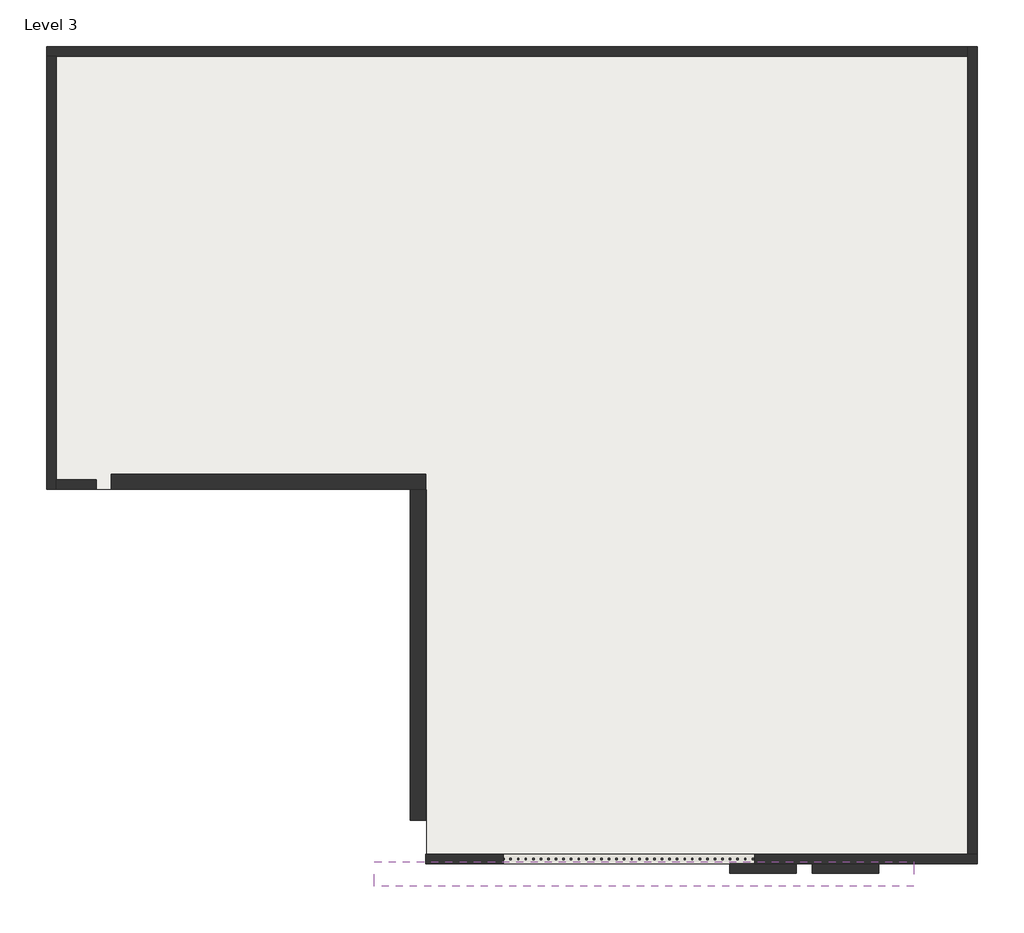
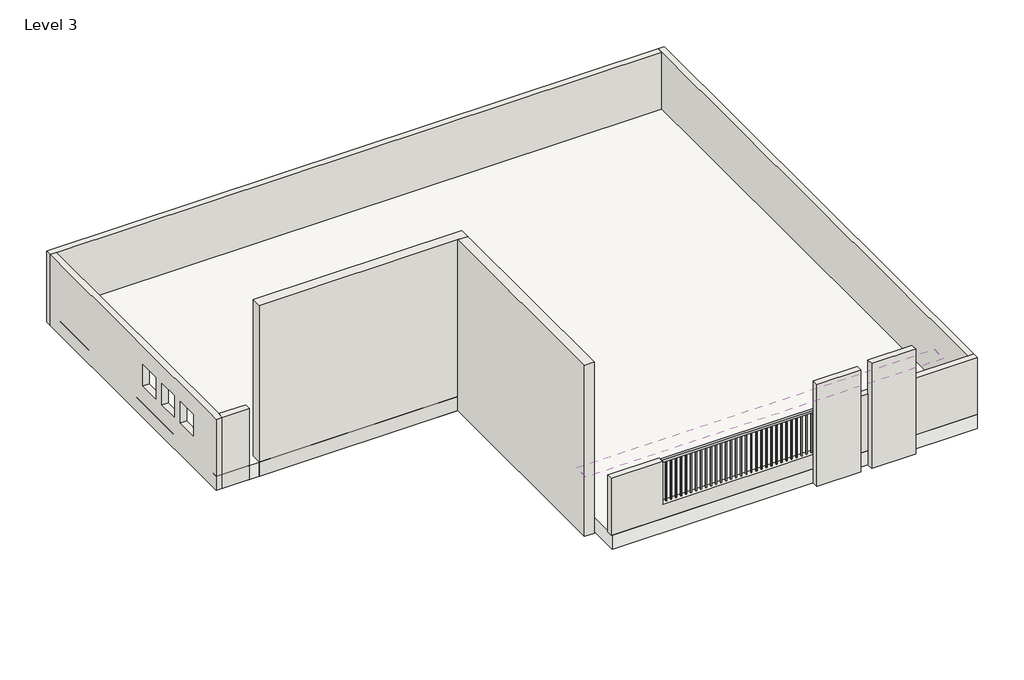
# One storey: 9 walls, 2 roofs, 1 railing.
"""IFC4 building model written with IfcOpenShell, lengths in millimetres."""

from ifc_helpers import new_model, si_unit, frame, origin, place, context, project, spatial, polyline, outline, extrude, faceted_brep, element, save

model = new_model("IFC4")

# Units and contexts
model_context = context("Model", 3, world=origin())
ifc_project = project(units=[si_unit("LENGTHUNIT", "METRE", prefix="MILLI")], contexts=[model_context])

# Site, building, storey
site = spatial("IfcSite", under=ifc_project)
building = spatial("IfcBuilding", under=site)
storey = spatial("IfcBuildingStorey", under=building, Name="Level 3", Elevation=7315.2)

# Railing
placement = place(None, origin())
element("IfcRailing", 1, ObjectType="Handrail - Rectangular", at=placement, inside=storey, context=model_context, shape_type="SweptSolid", body=[
    extrude(outline(polyline([(-6325.2932708, -2514.1516348), (-6325.2932708, -2463.3516348), (-2921.6932708, -2463.3516348), (-2921.6932708, -2514.1516348), (-6325.2932708, -2514.1516348)])), frame((0.0, 0.0, 8788.4), z_axis=(0.0, 0.0, 1.0), x_axis=(1.0, 0.0, 0.0)), (0.0, 0.0, 1.0), 50.8),
    extrude(outline(polyline([(-2982.0182708, -2498.2766348), (-2982.0182708, -2479.2266348), (-2962.9682708, -2479.2266348), (-2962.9682708, -2498.2766348), (-2982.0182708, -2498.2766348)])), frame((0.0, 0.0, 7924.8), z_axis=(0.0, 0.0, 1.0), x_axis=(1.0, 0.0, 0.0)), (0.0, 0.0, 1.0), 863.6),
    extrude(outline(polyline([(-3083.6182708, -2498.2766348), (-3083.6182708, -2479.2266348), (-3064.5682708, -2479.2266348), (-3064.5682708, -2498.2766348), (-3083.6182708, -2498.2766348)])), frame((0.0, 0.0, 7924.8), z_axis=(0.0, 0.0, 1.0), x_axis=(1.0, 0.0, 0.0)), (0.0, 0.0, 1.0), 863.6),
    extrude(outline(polyline([(-3185.2182708, -2498.2766348), (-3185.2182708, -2479.2266348), (-3166.1682708, -2479.2266348), (-3166.1682708, -2498.2766348), (-3185.2182708, -2498.2766348)])), frame((0.0, 0.0, 7924.8), z_axis=(0.0, 0.0, 1.0), x_axis=(1.0, 0.0, 0.0)), (0.0, 0.0, 1.0), 863.6),
    extrude(outline(polyline([(-3286.8182708, -2498.2766348), (-3286.8182708, -2479.2266348), (-3267.7682708, -2479.2266348), (-3267.7682708, -2498.2766348), (-3286.8182708, -2498.2766348)])), frame((0.0, 0.0, 7924.8), z_axis=(0.0, 0.0, 1.0), x_axis=(1.0, 0.0, 0.0)), (0.0, 0.0, 1.0), 863.6),
    extrude(outline(polyline([(-3388.4182708, -2498.2766348), (-3388.4182708, -2479.2266348), (-3369.3682708, -2479.2266348), (-3369.3682708, -2498.2766348), (-3388.4182708, -2498.2766348)])), frame((0.0, 0.0, 7924.8), z_axis=(0.0, 0.0, 1.0), x_axis=(1.0, 0.0, 0.0)), (0.0, 0.0, 1.0), 863.6),
    extrude(outline(polyline([(-3490.0182708, -2498.2766348), (-3490.0182708, -2479.2266348), (-3470.9682708, -2479.2266348), (-3470.9682708, -2498.2766348), (-3490.0182708, -2498.2766348)])), frame((0.0, 0.0, 7924.8), z_axis=(0.0, 0.0, 1.0), x_axis=(1.0, 0.0, 0.0)), (0.0, 0.0, 1.0), 863.6),
    extrude(outline(polyline([(-3591.6182708, -2498.2766348), (-3591.6182708, -2479.2266348), (-3572.5682708, -2479.2266348), (-3572.5682708, -2498.2766348), (-3591.6182708, -2498.2766348)])), frame((0.0, 0.0, 7924.8), z_axis=(0.0, 0.0, 1.0), x_axis=(1.0, 0.0, 0.0)), (0.0, 0.0, 1.0), 863.6),
    extrude(outline(polyline([(-3693.2182708, -2498.2766348), (-3693.2182708, -2479.2266348), (-3674.1682708, -2479.2266348), (-3674.1682708, -2498.2766348), (-3693.2182708, -2498.2766348)])), frame((0.0, 0.0, 7924.8), z_axis=(0.0, 0.0, 1.0), x_axis=(1.0, 0.0, 0.0)), (0.0, 0.0, 1.0), 863.6),
    extrude(outline(polyline([(-3794.8182708, -2498.2766348), (-3794.8182708, -2479.2266348), (-3775.7682708, -2479.2266348), (-3775.7682708, -2498.2766348), (-3794.8182708, -2498.2766348)])), frame((0.0, 0.0, 7924.8), z_axis=(0.0, 0.0, 1.0), x_axis=(1.0, 0.0, 0.0)), (0.0, 0.0, 1.0), 863.6),
    extrude(outline(polyline([(-3896.4182708, -2498.2766348), (-3896.4182708, -2479.2266348), (-3877.3682708, -2479.2266348), (-3877.3682708, -2498.2766348), (-3896.4182708, -2498.2766348)])), frame((0.0, 0.0, 7924.8), z_axis=(0.0, 0.0, 1.0), x_axis=(1.0, 0.0, 0.0)), (0.0, 0.0, 1.0), 863.6),
    extrude(outline(polyline([(-3998.0182708, -2498.2766348), (-3998.0182708, -2479.2266348), (-3978.9682708, -2479.2266348), (-3978.9682708, -2498.2766348), (-3998.0182708, -2498.2766348)])), frame((0.0, 0.0, 7924.8), z_axis=(0.0, 0.0, 1.0), x_axis=(1.0, 0.0, 0.0)), (0.0, 0.0, 1.0), 863.6),
    extrude(outline(polyline([(-4099.6182708, -2498.2766348), (-4099.6182708, -2479.2266348), (-4080.5682708, -2479.2266348), (-4080.5682708, -2498.2766348), (-4099.6182708, -2498.2766348)])), frame((0.0, 0.0, 7924.8), z_axis=(0.0, 0.0, 1.0), x_axis=(1.0, 0.0, 0.0)), (0.0, 0.0, 1.0), 863.6),
    extrude(outline(polyline([(-4201.2182708, -2498.2766348), (-4201.2182708, -2479.2266348), (-4182.1682708, -2479.2266348), (-4182.1682708, -2498.2766348), (-4201.2182708, -2498.2766348)])), frame((0.0, 0.0, 7924.8), z_axis=(0.0, 0.0, 1.0), x_axis=(1.0, 0.0, 0.0)), (0.0, 0.0, 1.0), 863.6),
    extrude(outline(polyline([(-4302.8182708, -2498.2766348), (-4302.8182708, -2479.2266348), (-4283.7682708, -2479.2266348), (-4283.7682708, -2498.2766348), (-4302.8182708, -2498.2766348)])), frame((0.0, 0.0, 7924.8), z_axis=(0.0, 0.0, 1.0), x_axis=(1.0, 0.0, 0.0)), (0.0, 0.0, 1.0), 863.6),
    extrude(outline(polyline([(-4404.4182708, -2498.2766348), (-4404.4182708, -2479.2266348), (-4385.3682708, -2479.2266348), (-4385.3682708, -2498.2766348), (-4404.4182708, -2498.2766348)])), frame((0.0, 0.0, 7924.8), z_axis=(0.0, 0.0, 1.0), x_axis=(1.0, 0.0, 0.0)), (0.0, 0.0, 1.0), 863.6),
    extrude(outline(polyline([(-4506.0182708, -2498.2766348), (-4506.0182708, -2479.2266348), (-4486.9682708, -2479.2266348), (-4486.9682708, -2498.2766348), (-4506.0182708, -2498.2766348)])), frame((0.0, 0.0, 7924.8), z_axis=(0.0, 0.0, 1.0), x_axis=(1.0, 0.0, 0.0)), (0.0, 0.0, 1.0), 863.6),
    extrude(outline(polyline([(-4607.6182708, -2498.2766348), (-4607.6182708, -2479.2266348), (-4588.5682708, -2479.2266348), (-4588.5682708, -2498.2766348), (-4607.6182708, -2498.2766348)])), frame((0.0, 0.0, 7924.8), z_axis=(0.0, 0.0, 1.0), x_axis=(1.0, 0.0, 0.0)), (0.0, 0.0, 1.0), 863.6),
    extrude(outline(polyline([(-4709.2182708, -2498.2766348), (-4709.2182708, -2479.2266348), (-4690.1682708, -2479.2266348), (-4690.1682708, -2498.2766348), (-4709.2182708, -2498.2766348)])), frame((0.0, 0.0, 7924.8), z_axis=(0.0, 0.0, 1.0), x_axis=(1.0, 0.0, 0.0)), (0.0, 0.0, 1.0), 863.6),
    extrude(outline(polyline([(-4810.8182708, -2498.2766348), (-4810.8182708, -2479.2266348), (-4791.7682708, -2479.2266348), (-4791.7682708, -2498.2766348), (-4810.8182708, -2498.2766348)])), frame((0.0, 0.0, 7924.8), z_axis=(0.0, 0.0, 1.0), x_axis=(1.0, 0.0, 0.0)), (0.0, 0.0, 1.0), 863.6),
    extrude(outline(polyline([(-4912.4182708, -2498.2766348), (-4912.4182708, -2479.2266348), (-4893.3682708, -2479.2266348), (-4893.3682708, -2498.2766348), (-4912.4182708, -2498.2766348)])), frame((0.0, 0.0, 7924.8), z_axis=(0.0, 0.0, 1.0), x_axis=(1.0, 0.0, 0.0)), (0.0, 0.0, 1.0), 863.6),
    extrude(outline(polyline([(-5014.0182708, -2498.2766348), (-5014.0182708, -2479.2266348), (-4994.9682708, -2479.2266348), (-4994.9682708, -2498.2766348), (-5014.0182708, -2498.2766348)])), frame((0.0, 0.0, 7924.8), z_axis=(0.0, 0.0, 1.0), x_axis=(1.0, 0.0, 0.0)), (0.0, 0.0, 1.0), 863.6),
    extrude(outline(polyline([(-5115.6182708, -2498.2766348), (-5115.6182708, -2479.2266348), (-5096.5682708, -2479.2266348), (-5096.5682708, -2498.2766348), (-5115.6182708, -2498.2766348)])), frame((0.0, 0.0, 7924.8), z_axis=(0.0, 0.0, 1.0), x_axis=(1.0, 0.0, 0.0)), (0.0, 0.0, 1.0), 863.6),
    extrude(outline(polyline([(-5217.2182708, -2498.2766348), (-5217.2182708, -2479.2266348), (-5198.1682708, -2479.2266348), (-5198.1682708, -2498.2766348), (-5217.2182708, -2498.2766348)])), frame((0.0, 0.0, 7924.8), z_axis=(0.0, 0.0, 1.0), x_axis=(1.0, 0.0, 0.0)), (0.0, 0.0, 1.0), 863.6),
    extrude(outline(polyline([(-5318.8182708, -2498.2766348), (-5318.8182708, -2479.2266348), (-5299.7682708, -2479.2266348), (-5299.7682708, -2498.2766348), (-5318.8182708, -2498.2766348)])), frame((0.0, 0.0, 7924.8), z_axis=(0.0, 0.0, 1.0), x_axis=(1.0, 0.0, 0.0)), (0.0, 0.0, 1.0), 863.6),
    extrude(outline(polyline([(-5420.4182708, -2498.2766348), (-5420.4182708, -2479.2266348), (-5401.3682708, -2479.2266348), (-5401.3682708, -2498.2766348), (-5420.4182708, -2498.2766348)])), frame((0.0, 0.0, 7924.8), z_axis=(0.0, 0.0, 1.0), x_axis=(1.0, 0.0, 0.0)), (0.0, 0.0, 1.0), 863.6),
    extrude(outline(polyline([(-5522.0182708, -2498.2766348), (-5522.0182708, -2479.2266348), (-5502.9682708, -2479.2266348), (-5502.9682708, -2498.2766348), (-5522.0182708, -2498.2766348)])), frame((0.0, 0.0, 7924.8), z_axis=(0.0, 0.0, 1.0), x_axis=(1.0, 0.0, 0.0)), (0.0, 0.0, 1.0), 863.6),
    extrude(outline(polyline([(-5623.6182708, -2498.2766348), (-5623.6182708, -2479.2266348), (-5604.5682708, -2479.2266348), (-5604.5682708, -2498.2766348), (-5623.6182708, -2498.2766348)])), frame((0.0, 0.0, 7924.8), z_axis=(0.0, 0.0, 1.0), x_axis=(1.0, 0.0, 0.0)), (0.0, 0.0, 1.0), 863.6),
    extrude(outline(polyline([(-5725.2182708, -2498.2766348), (-5725.2182708, -2479.2266348), (-5706.1682708, -2479.2266348), (-5706.1682708, -2498.2766348), (-5725.2182708, -2498.2766348)])), frame((0.0, 0.0, 7924.8), z_axis=(0.0, 0.0, 1.0), x_axis=(1.0, 0.0, 0.0)), (0.0, 0.0, 1.0), 863.6),
    extrude(outline(polyline([(-5826.8182708, -2498.2766348), (-5826.8182708, -2479.2266348), (-5807.7682708, -2479.2266348), (-5807.7682708, -2498.2766348), (-5826.8182708, -2498.2766348)])), frame((0.0, 0.0, 7924.8), z_axis=(0.0, 0.0, 1.0), x_axis=(1.0, 0.0, 0.0)), (0.0, 0.0, 1.0), 863.6),
    extrude(outline(polyline([(-5928.4182708, -2498.2766348), (-5928.4182708, -2479.2266348), (-5909.3682708, -2479.2266348), (-5909.3682708, -2498.2766348), (-5928.4182708, -2498.2766348)])), frame((0.0, 0.0, 7924.8), z_axis=(0.0, 0.0, 1.0), x_axis=(1.0, 0.0, 0.0)), (0.0, 0.0, 1.0), 863.6),
    extrude(outline(polyline([(-6030.0182708, -2498.2766348), (-6030.0182708, -2479.2266348), (-6010.9682708, -2479.2266348), (-6010.9682708, -2498.2766348), (-6030.0182708, -2498.2766348)])), frame((0.0, 0.0, 7924.8), z_axis=(0.0, 0.0, 1.0), x_axis=(1.0, 0.0, 0.0)), (0.0, 0.0, 1.0), 863.6),
    extrude(outline(polyline([(-6131.6182708, -2498.2766348), (-6131.6182708, -2479.2266348), (-6112.5682708, -2479.2266348), (-6112.5682708, -2498.2766348), (-6131.6182708, -2498.2766348)])), frame((0.0, 0.0, 7924.8), z_axis=(0.0, 0.0, 1.0), x_axis=(1.0, 0.0, 0.0)), (0.0, 0.0, 1.0), 863.6),
    extrude(outline(polyline([(-6233.2182708, -2498.2766348), (-6233.2182708, -2479.2266348), (-6214.1682708, -2479.2266348), (-6214.1682708, -2498.2766348), (-6233.2182708, -2498.2766348)])), frame((0.0, 0.0, 7924.8), z_axis=(0.0, 0.0, 1.0), x_axis=(1.0, 0.0, 0.0)), (0.0, 0.0, 1.0), 863.6),
    extrude(outline(polyline([(-2940.7432708, -2498.2766348), (-2940.7432708, -2479.2266348), (-2921.6932708, -2479.2266348), (-2921.6932708, -2498.2766348), (-2940.7432708, -2498.2766348)])), frame((0.0, 0.0, 7924.8), z_axis=(0.0, 0.0, 1.0), x_axis=(1.0, 0.0, 0.0)), (0.0, 0.0, 1.0), 863.6),
    extrude(outline(polyline([(-6325.2932708, -2498.2766348), (-6325.2932708, -2479.2266348), (-6306.2432708, -2479.2266348), (-6306.2432708, -2498.2766348), (-6325.2932708, -2498.2766348)])), frame((0.0, 0.0, 7924.8), z_axis=(0.0, 0.0, 1.0), x_axis=(1.0, 0.0, 0.0)), (0.0, 0.0, 1.0), 863.6),
])

# Roofs
element("IfcRoof", 2, ObjectType="Generic - 12\"", at=placement, inside=storey, context=model_context, shape_type="SweptSolid", body=[
    extrude(outline(polyline([(-12453.9083357, 8420.5483652), (42.8916643, 8420.5483652), (42.8916643, -2552.2516348), (-7348.5083357, -2552.2516348), (-7348.5083357, 2476.9483652), (-12453.9083357, 2476.9483652), (-12453.9083357, 8420.5483652)])), frame((0.0, 0.0, 7315.2), z_axis=(0.0, 0.0, 1.0), x_axis=(1.0, 0.0, 0.0)), (0.0, 0.0, 1.0), 304.8),
])
element("IfcRoof", 3, ObjectType="Generic - 12\"", at=placement, inside=storey, context=model_context, shape_type="SweptSolid", body=[
    extrude(outline(polyline([(-8052.4932708, -2521.726099), (-813.4932708, -2521.726099), (-813.4932708, -2853.7303933), (-8052.4932708, -2853.7303933), (-8052.4932708, -2521.726099)])), frame((0.0, 0.0, 9296.4), z_axis=(0.0, 0.0, 1.0), x_axis=(1.0, 0.0, 0.0)), (0.0, 0.0, 1.0), 304.8),
])

# Walls
element("IfcWall", 4, ObjectType="Generic - 5\"", at=placement, inside=storey, context=model_context, shape_type="Brep", body=[
    faceted_brep([(42.8916643, -2425.2516348, 7620.0), (-7366.6932708, -2425.2516348, 7620.0), (-7366.6932708, -2425.2516348, 8839.2), (-6325.2932708, -2425.2516348, 8839.2), (-6325.2932708, -2425.2516348, 7924.8), (-2949.0420604, -2425.2516348, 7924.8), (-2949.0420604, -2425.2516348, 8839.2), (-84.1083357, -2425.2516348, 8839.2), (42.8916643, -2425.2516348, 8839.2), (42.8916643, -2552.2516348, 7620.0), (42.8916643, -2552.2516348, 8839.2), (-2949.0420604, -2552.2516348, 8839.2), (-2949.0420604, -2552.2516348, 7924.8), (-6325.2932708, -2552.2516348, 7924.8), (-6325.2932708, -2552.2516348, 8839.2), (-7366.6932708, -2552.2516348, 8839.2), (-7366.6932708, -2552.2516348, 7620.0)], [[[0, 1, 2, 3, 4, 5, 6, 7, 8]], [[9, 10, 11, 12, 13, 14, 15, 16]], [[2, 1, 16, 15]], [[0, 8, 10, 9]], [[1, 0, 9, 16]], [[3, 2, 15, 14]], [[4, 3, 14, 13]], [[5, 4, 13, 12]], [[6, 5, 12, 11]], [[8, 7, 6, 11, 10]]]),
])
element("IfcWall", 5, ObjectType="Generic - 5\"", at=placement, inside=storey, context=model_context, shape_type="Brep", body=[
    faceted_brep([(42.8916643, -2425.2516348, 7315.2), (42.8916643, 8420.5483652, 7315.2), (42.8916643, 8420.5483652, 8839.2), (42.8916643, -2425.2516348, 8839.2), (42.8916643, -2425.2516348, 7620.0), (-84.1083357, -2425.2516348, 7315.2), (-84.1083357, -2425.2516348, 8839.2), (-84.1083357, 8293.5483652, 8839.2), (-84.1083357, 8420.5483652, 8839.2), (-84.1083357, 8420.5483652, 7315.2), (-84.1083357, 8293.5483652, 7315.2)], [[[0, 1, 2, 3, 4]], [[5, 6, 7, 8, 9, 10]], [[1, 0, 5, 10, 9]], [[3, 2, 8, 7, 6]], [[0, 4, 3, 6, 5]], [[2, 1, 9, 8]]]),
])
element("IfcWall", 6, ObjectType="Generic - 5\"", at=placement, inside=storey, context=model_context, shape_type="Brep", body=[
    faceted_brep([(-84.1083357, 8420.5483652, 7315.2), (-12453.9083357, 8420.5483652, 7315.2), (-12453.9083357, 8420.5483652, 8839.2), (-84.1083357, 8420.5483652, 8839.2), (-84.1083357, 8293.5483652, 7315.2), (-84.1083357, 8293.5483652, 8839.2), (-12326.9083357, 8293.5483652, 8839.2), (-12453.9083357, 8293.5483652, 8839.2), (-12453.9083357, 8293.5483652, 7315.2), (-12326.9083357, 8293.5483652, 7315.2)], [[[0, 1, 2, 3]], [[4, 5, 6, 7, 8, 9]], [[1, 0, 4, 9, 8]], [[3, 2, 7, 6, 5]], [[0, 3, 5, 4]], [[2, 1, 8, 7]]]),
])
element("IfcWall", 7, ObjectType="Generic - 5\"", at=placement, inside=storey, context=model_context, shape_type="Brep", body=[
    faceted_brep([(-12453.9083357, 8293.5483652, 7315.2), (-12453.9083357, 2476.9483652, 7315.2), (-12453.9083357, 2476.9483652, 8839.2), (-12453.9083357, 8293.5483652, 8839.2), (-12453.9083357, 4589.1211472, 8455.5035139), (-12453.9083357, 4589.1211472, 7998.3035139), (-12453.9083357, 5046.3211472, 7998.3035139), (-12453.9083357, 5046.3211472, 8455.5035139), (-12453.9083357, 3946.3457143, 8455.5035139), (-12453.9083357, 3946.3457143, 7998.3035139), (-12453.9083357, 4376.7708837, 7998.3035139), (-12453.9083357, 4376.7708837, 8455.5035139), (-12453.9083357, 3283.3854734, 8455.5035139), (-12453.9083357, 3283.3854734, 7998.3035139), (-12453.9083357, 3732.9406503, 7998.3035139), (-12453.9083357, 3732.9406503, 8455.5035139), (-12326.9083357, 8293.5483652, 7315.2), (-12326.9083357, 8293.5483652, 8839.2), (-12326.9083357, 2603.9483652, 8839.2), (-12326.9083357, 2476.9483652, 8839.2), (-12326.9083357, 2476.9483652, 7315.2), (-12326.9083357, 2603.9483652, 7315.2), (-12326.9083357, 4589.1211472, 8455.5035139), (-12326.9083357, 5046.3211472, 8455.5035139), (-12326.9083357, 5046.3211472, 7998.3035139), (-12326.9083357, 4589.1211472, 7998.3035139), (-12326.9083357, 3946.3457143, 8455.5035139), (-12326.9083357, 4376.7708837, 8455.5035139), (-12326.9083357, 4376.7708837, 7998.3035139), (-12326.9083357, 3946.3457143, 7998.3035139), (-12326.9083357, 3283.3854734, 8455.5035139), (-12326.9083357, 3732.9406503, 8455.5035139), (-12326.9083357, 3732.9406503, 7998.3035139), (-12326.9083357, 3283.3854734, 7998.3035139)], [[[0, 1, 2, 3], [4, 5, 6, 7], [8, 9, 10, 11], [12, 13, 14, 15]], [[16, 17, 18, 19, 20, 21], [22, 23, 24, 25], [26, 27, 28, 29], [30, 31, 32, 33]], [[0, 3, 17, 16]], [[2, 1, 20, 19]], [[1, 0, 16, 21, 20]], [[3, 2, 19, 18, 17]], [[5, 4, 22, 25]], [[6, 5, 25, 24]], [[7, 6, 24, 23]], [[4, 7, 23, 22]], [[9, 8, 26, 29]], [[10, 9, 29, 28]], [[11, 10, 28, 27]], [[8, 11, 27, 26]], [[13, 12, 30, 33]], [[14, 13, 33, 32]], [[15, 14, 32, 31]], [[12, 15, 31, 30]]]),
])
element("IfcWall", 8, ObjectType="Generic - 5\"", at=placement, inside=storey, context=model_context, shape_type="SweptSolid", body=[
    extrude(outline(polyline([(-11786.2932708, 2476.9483652), (-12326.9083357, 2476.9483652), (-12326.9083357, 2603.9483652), (-11786.2932708, 2603.9483652), (-11786.2932708, 2476.9483652)])), frame((0.0, 0.0, 7315.2), z_axis=(0.0, 0.0, 1.0), x_axis=(1.0, 0.0, 0.0)), (0.0, 0.0, 1.0), 1524.0),
])
element("IfcWall", 9, ObjectType="Generic - 5\"", at=placement, inside=storey, context=model_context, shape_type="SweptSolid", body=[
    extrude(outline(polyline([(-2390.2420604, -2679.2516348), (-3279.2420604, -2679.2516348), (-3279.2420604, -2552.2516348), (-2390.2420604, -2552.2516348), (-2390.2420604, -2679.2516348)])), frame((0.0, 0.0, 7315.2), z_axis=(0.0, 0.0, 1.0), x_axis=(1.0, 0.0, 0.0)), (0.0, 0.0, 1.0), 2186.3186907),
])
element("IfcWall", 10, ObjectType="Generic - 5\"", at=placement, inside=storey, context=model_context, shape_type="SweptSolid", body=[
    extrude(outline(polyline([(-2172.3932708, -2552.2516348), (-1283.3932708, -2552.2516348), (-1283.3932708, -2679.2516348), (-2172.3932708, -2679.2516348), (-2172.3932708, -2552.2516348)])), frame((0.0, 0.0, 7315.2), z_axis=(0.0, 0.0, 1.0), x_axis=(1.0, 0.0, 0.0)), (0.0, 0.0, 1.0), 2243.0287149),
])
element("IfcWall", 11, ObjectType="Generic - 8\"", at=placement, inside=storey, context=model_context, shape_type="Brep", body=[
    faceted_brep([(-11583.0932708, 2476.9483652, 10972.8), (-11583.0932708, 2476.9483652, 7315.2), (-7569.8932708, 2476.9483652, 7315.2), (-7366.6932708, 2476.9483652, 7315.2), (-7366.6932708, 2476.9483652, 10972.8), (-7569.8932708, 2476.9483652, 10972.8), (-11583.0932708, 2680.1483652, 7315.2), (-11583.0932708, 2680.1483652, 10972.8), (-7366.6932708, 2680.1483652, 10972.8), (-7366.6932708, 2680.1483652, 7315.2)], [[[0, 1, 2, 3, 4, 5]], [[6, 7, 8, 9]], [[3, 2, 1, 6, 9]], [[4, 3, 9, 8]], [[0, 5, 4, 8, 7]], [[0, 7, 6, 1]]]),
])
element("IfcWall", 12, ObjectType="Generic - 8\"", at=placement, inside=storey, context=model_context, shape_type="Brep", body=[
    faceted_brep([(-7366.6932708, -1962.926099, 7315.2), (-7366.6932708, -1861.326099, 7315.2), (-7366.6932708, 2476.9483652, 7315.2), (-7366.6932708, 2476.9483652, 10972.8), (-7366.6932708, -1962.926099, 10972.8), (-7569.8932708, -1962.926099, 7315.2), (-7569.8932708, -1962.926099, 10972.8), (-7569.8932708, 2476.9483652, 10972.8), (-7569.8932708, 2476.9483652, 7315.2), (-7569.8932708, -1861.326099, 7315.2)], [[[0, 1, 2, 3, 4]], [[5, 6, 7, 8, 9]], [[2, 1, 0, 5, 9, 8]], [[4, 3, 7, 6]], [[0, 4, 6, 5]], [[3, 2, 8, 7]]]),
])

save(model, "model.ifc")

# Revit data of these elements
# Type "Handrail - Rectangular"
#   Assembly Code = "C2010400"
#   built-in parameter 1008612 = 0.0416667 (stored number, unit not read)
#   built-in parameter 1008611 = 0.0416667 (stored number, unit not read)
#   built-in parameter 1008609 = 0.333333 (stored number, unit not read)
#   built-in parameter 1008604 = 0.166667 (stored number, unit not read)
#   built-in parameter 1008603 = 0.166667 (stored number, unit not read)
#   Railing Height = 3' - 0"
#   built-in parameter 1008630 = 2
#   built-in parameter 1008610 = 2
#   built-in parameter 1008618 = Baluster - Square : 3/4"
# Type "Generic - 12\""
#   Assembly Code = "B1020"
#   Layers, outside or top first: 1' - 0" no material (function 1)
# Type "Generic - 5\""
#   Assembly Code = "B2010"
#   Layers, outside or top first: 0' - 5" no material (function 1)
# Type "Generic - 8\""
#   Assembly Code = "B2010"
#   Layers, outside or top first: 0' - 8" no material (function 1)
# Element 1 (IfcRailing, "Handrail - Rectangular")
#   built-in parameter 1008621 = 2 (stored number, unit not read)
#   Phase Created = New Construction
# Element 2 (IfcRoof, "Generic - 12\"")
#   built-in parameter 1001705 = 25 (stored number, unit not read)
#   built-in parameter 1001710 = 33615
#   Phase Created = New Construction
#   Materials on its faces: "Default Roof"
# Element 3 (IfcRoof, "Generic - 12\"")
#   built-in parameter 1001705 = 31.5 (stored number, unit not read)
#   built-in parameter 1001701 = 6.5 (stored number, unit not read)
#   built-in parameter 1001710 = 33615
#   Phase Created = New Construction
#   Materials on its faces: "Default Roof"
# Element 4 (IfcWall, "Generic - 5\"")
#   built-in parameter 1001111 = 1' - 0"
#   Top Offset = -7' - 0"
#   Base Offset = 1' - 0"
#   wall height = 4' - 0"
#   Phase Created = New Construction
#   Base Constraint = Level 3
#   Top Constraint = Level 4
#   Materials on its faces: "Default Wall"
# Elements 5, 6, 7, 8 (IfcWall, "Generic - 5\"")
#   Top Offset = -7' - 0"
#   Base Offset = 0' - 0"
#   wall height = 5' - 0"
#   Phase Created = New Construction
#   Base Constraint = Level 3
#   Top Constraint = Level 4
#   Materials on its faces: "Default Wall"
# Element 9 (IfcWall, "Generic - 5\"")
#   Top Offset = -4' - 9.92446"
#   Base Offset = 0' - 0"
#   wall height = 7' - 2.07554"
#   Phase Created = New Construction
#   Base Constraint = Level 3
#   Top Constraint = Level 4
#   Materials on its faces: "Default Wall"
# Element 10 (IfcWall, "Generic - 5\"")
#   Top Offset = -4' - 7.69178"
#   Base Offset = 0' - 0"
#   wall height = 7' - 4.30822"
#   Phase Created = New Construction
#   Base Constraint = Level 3
#   Top Constraint = Level 4
#   Materials on its faces: "Default Wall"
# Elements 11, 12 (IfcWall, "Generic - 8\"")
#   Top Offset = 0' - 0"
#   Base Offset = 0' - 0"
#   Unconnected Height = 12' - 0"
#   wall height = 12' - 0"
#   Phase Created = New Construction
#   Base Constraint = Level 3
#   Materials on its faces: "Default Wall"
# Materials
#   "Default Roof": colour RGB 88 101 114, transparency 0
#   "Default Wall": colour RGB 128 128 128, transparency 0
